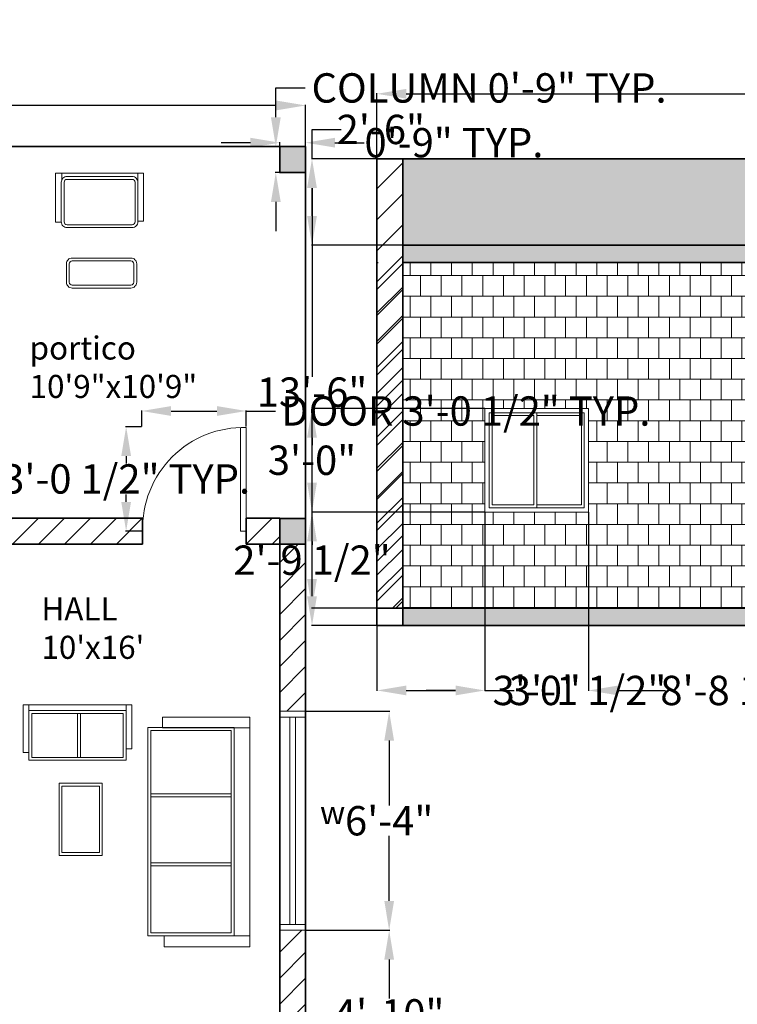
# Model space of a CAD drawing. Units: inches. Extents: x 1222 to 2611, y 176 to 793.
# Tile 3 of 5: x 1497 to 1746, y 433 to 775. Entities that reach past the tile are written whole.
import ezdxf

# ---------------------------------------------------------------- set-up
doc = ezdxf.new("R2010")
doc.units = ezdxf.units.IN
doc.header["$MEASUREMENT"] = 0
for name, color, linetype, lineweight in [('A-ANNO-DIMS', 2, 'Continuous', 18), ('A-ANNO-TEXT', 7, 'Continuous', 25), ('A-AREA-IDEN', 7, 'Continuous', 25), ('A-COLS', 7, 'Continuous', 35), ('A-COLS-PATT', 18, 'Continuous', 13), ('A-DOOR', 3, 'Continuous', 18), ('A-ELEV', 7, 'Continuous', 35), ('A-ELEV-GLAZ', 4, 'Continuous', 18), ('A-ELEV-PATT', 30, 'Continuous', 13), ('A-FURN', 8, 'Continuous', 18), ('A-GLAZ', 4, 'Continuous', 18), ('A-WALL', 7, 'Continuous', 35), ('A-WALL-PATT', 30, 'Continuous', 13)]:
    doc.layers.add(name, color=color, linetype=linetype, lineweight=lineweight)
doc.styles.get("Standard").update_dxf_attribs({"font": 'arial.ttf'})
doc.dimstyles.get("Standard").update_dxf_attribs({"dimtxt": 10.18, "dimasz": 10.18, "dimexe": 0.18, "dimexo": 0.0625, "dimgap": 0.09, "dimtad": 0, "dimtih": 1, "dimtoh": 1, "dimdec": 0, "dimzin": 0, "dimdsep": 46, "dimlunit": 3, "dimtxsty": 'Standard', "dimcen": 0.09, "dimadec": 0, "dimazin": 0, "dimtfac": 1, "dimtdec": 0, "dimtofl": 0, "dimtmove": 0, "dimatfit": 3, "dimfxl": 1, "dimtolj": 1, "dimtzin": 0, "dimarcsym": 0})

# ---------------------------------------------------------------- blocks, each defined once
blk = doc.blocks.new('*U6')
for p, q in [((1.5, 1.5), (1.5, 34.5)), ((1.5, 34.5), (18, 34.5)), ((18, 1.5), (18, 34.5)), ((18, 34.5), (34.5, 34.5)), ((34.5, 34.5), (34.5, 1.5)), ((18, 1.5), (1.5, 1.5)), ((34.5, 1.5), (18, 1.5))]:
    blk.add_line(p, q)
blk.add_lwpolyline([(0, 0), (0, 36), (36, 36), (36, 0)], close=True)
for points in [[(17, 33.5), (17, 2.5), (2.5, 2.5), (2.5, 33.5), (17, 33.5)], [(18, 33.5), (33.5, 33.5), (33.5, 2.5), (18, 2.5)]]:
    blk.add_lwpolyline(points)
blk = doc.blocks.new('*D9')
at = {"layer": 'A-ANNO-DIMS', "color": 0, "lineweight": -2, "transparency": 16777216}
for p, q in [((1328.8, 730.54), (1328.8, 744.93)), ((1338.98, 744.75), (1444.64, 744.75)), ((1585.62, 744.75), (1479.97, 744.75)), ((1595.8, 730.54), (1595.8, 744.93))]:
    blk.add_line(p, q, dxfattribs=at)
at = {"layer": 'A-ANNO-DIMS', "color": 0, "transparency": 16777216}
for points in [[(1338.98, 746.45), (1338.98, 743.05), (1328.8, 744.75)], [(1585.62, 746.45), (1585.62, 743.05), (1595.8, 744.75)]]:
    blk.add_solid(points, dxfattribs=at)
at = {"layer": 'Defpoints', "color": 0, "transparency": 16777216}
for p in [(1595.8, 744.75), (1328.8, 730.47), (1595.8, 730.47)]:
    blk.add_point(p, dxfattribs=at)
at = {"layer": 'A-ANNO-DIMS', "color": 0, "transparency": 16777216, "insert": (1462.3, 744.75), "char_height": 10.18, "attachment_point": 5}
blk.add_mtext('\\A1;22\'-3"', dxfattribs=at)
blk = doc.blocks.new('DOOR-SWING-36IN')
for p, q in [((34.01, 0), (34.01, 36)), ((36.01, 0), (36.01, 36)), ((34.01, 0), (36.01, 0))]:
    blk.add_line(p, q)
blk.add_arc((35.01, 1), 35.01, 88.3634, 181.6366)
blk = doc.blocks.new('COLUMN-9X9IN')
blk.add_lwpolyline([(0, 9), (9, 9), (9, 0), (0, 0)], close=True)
blk = doc.blocks.new('*D16')
at = {"layer": 'A-ANNO-DIMS', "color": 0, "lineweight": -2, "transparency": 16777216}
for p, q in [((1585.45, 740.65), (1585.45, 750.83)), ((1585.45, 750.83), (1595.63, 750.83)), ((1586.74, 730.47), (1585.27, 730.47)), ((1586.74, 721.47), (1585.27, 721.47)), ((1585.45, 711.29), (1585.45, 701.11))]:
    blk.add_line(p, q, dxfattribs=at)
at = {"layer": 'A-ANNO-DIMS', "color": 0, "transparency": 16777216}
for points in [[(1583.76, 740.65), (1587.15, 740.65), (1585.45, 730.47)], [(1583.76, 711.29), (1587.15, 711.29), (1585.45, 721.47)]]:
    blk.add_solid(points, dxfattribs=at)
at = {"layer": 'Defpoints', "color": 0, "transparency": 16777216}
for p in [(1585.45, 730.47), (1586.8, 730.47), (1586.8, 721.47)]:
    blk.add_point(p, dxfattribs=at)
at = {"layer": 'A-ANNO-DIMS', "color": 0, "transparency": 16777216, "insert": (1659.48, 750.83), "char_height": 10.18, "attachment_point": 5}
blk.add_mtext('\\A1;COLUMN 0\'-9" TYP.', dxfattribs=at)
blk = doc.blocks.new('*D17')
at = {"layer": 'A-ANNO-DIMS', "color": 0, "lineweight": -2, "transparency": 16777216}
for p, q in [((1576.62, 731.82), (1566.44, 731.82)), ((1586.8, 730.54), (1586.8, 732)), ((1595.8, 730.54), (1595.8, 732)), ((1605.98, 731.82), (1616.16, 731.82))]:
    blk.add_line(p, q, dxfattribs=at)
at = {"layer": 'A-ANNO-DIMS', "color": 0, "transparency": 16777216}
for points in [[(1576.62, 733.52), (1576.62, 730.13), (1586.8, 731.82)], [(1605.98, 733.52), (1605.98, 730.13), (1595.8, 731.82)]]:
    blk.add_solid(points, dxfattribs=at)
at = {"layer": 'Defpoints', "color": 0, "transparency": 16777216}
for p in [(1595.8, 731.82), (1586.8, 730.47), (1595.8, 730.47)]:
    blk.add_point(p, dxfattribs=at)
at = {"layer": 'A-ANNO-DIMS', "color": 0, "transparency": 16777216, "insert": (1647.28, 731.82), "char_height": 10.18, "attachment_point": 5}
blk.add_mtext('\\A1;0\'-9" TYP.', dxfattribs=at)
blk = doc.blocks.new('*D20')
at = {"layer": 'A-ANNO-DIMS', "color": 0, "lineweight": -2, "transparency": 16777216}
for p, q in [((1538.92, 633.31), (1538.92, 638.87)), ((1549.1, 638.69), (1565.02, 638.69)), ((1575.2, 633.31), (1575.2, 638.87)), ((1575.2, 638.69), (1585.38, 638.69))]:
    blk.add_line(p, q, dxfattribs=at)
at = {"layer": 'A-ANNO-DIMS', "color": 0, "transparency": 16777216}
for points in [[(1549.1, 640.39), (1549.1, 636.99), (1538.92, 638.69)], [(1565.02, 640.39), (1565.02, 636.99), (1575.2, 638.69)]]:
    blk.add_solid(points, dxfattribs=at)
at = {"layer": 'Defpoints', "color": 0, "transparency": 16777216}
for p in [(1575.2, 638.69), (1538.92, 633.25), (1575.2, 633.25)]:
    blk.add_point(p, dxfattribs=at)
at = {"layer": 'A-ANNO-DIMS', "color": 0, "transparency": 16777216, "insert": (1651.41, 638.69), "char_height": 10.18, "attachment_point": 5}
blk.add_mtext('\\A1;DOOR 3\'-0 1/2" TYP.', dxfattribs=at)
blk = doc.blocks.new('*D21')
at = {"layer": 'A-ANNO-DIMS', "color": 0, "lineweight": -2, "transparency": 16777216}
for p, q in [((1538.86, 633.25), (1533.3, 633.25)), ((1533.48, 623.07), (1533.48, 620.47)), ((1533.48, 607.15), (1533.48, 609.75)), ((1538.86, 596.97), (1533.3, 596.97))]:
    blk.add_line(p, q, dxfattribs=at)
at = {"layer": 'A-ANNO-DIMS', "color": 0, "transparency": 16777216}
for points in [[(1531.79, 623.07), (1535.18, 623.07), (1533.48, 633.25)], [(1531.79, 607.15), (1535.18, 607.15), (1533.48, 596.97)]]:
    blk.add_solid(points, dxfattribs=at)
at = {"layer": 'Defpoints', "color": 0, "transparency": 16777216}
for p in [(1533.48, 633.25), (1538.92, 633.25), (1538.92, 596.97)]:
    blk.add_point(p, dxfattribs=at)
at = {"layer": 'A-ANNO-DIMS', "color": 0, "transparency": 16777216, "insert": (1533.48, 615.11), "char_height": 10.18, "attachment_point": 5}
blk.add_mtext('\\A1;3\'-0 1/2" TYP.', dxfattribs=at)
blk = doc.blocks.new('*D36')
at = {"layer": 'A-ANNO-DIMS', "color": 0, "lineweight": -2, "transparency": 16777216}
for p, q in [((1595.87, 458.47), (1624.98, 458.47)), ((1624.8, 448.29), (1624.8, 434.73)), ((1624.8, 410.59), (1624.8, 424.15)), ((1595.87, 400.41), (1624.98, 400.41))]:
    blk.add_line(p, q, dxfattribs=at)
at = {"layer": 'A-ANNO-DIMS', "color": 0, "transparency": 16777216}
for points in [[(1623.11, 448.29), (1626.5, 448.29), (1624.8, 458.47)], [(1623.11, 410.59), (1626.5, 410.59), (1624.8, 400.41)]]:
    blk.add_solid(points, dxfattribs=at)
at = {"layer": 'Defpoints', "color": 0, "transparency": 16777216}
for p in [(1595.8, 458.47), (1624.8, 458.47), (1595.8, 400.41)]:
    blk.add_point(p, dxfattribs=at)
at = {"layer": 'A-ANNO-DIMS', "color": 0, "transparency": 16777216, "insert": (1624.8, 429.44), "char_height": 10.18, "attachment_point": 5}
blk.add_mtext('\\A1;4\'-10"', dxfattribs=at)
blk = doc.blocks.new('*D37')
at = {"layer": 'A-ANNO-DIMS', "color": 0, "lineweight": -2, "transparency": 16777216}
for p, q in [((1595.87, 534.47), (1624.98, 534.47)), ((1624.8, 524.29), (1624.8, 501.76)), ((1624.8, 468.65), (1624.8, 491.19)), ((1595.87, 458.47), (1624.98, 458.47))]:
    blk.add_line(p, q, dxfattribs=at)
at = {"layer": 'A-ANNO-DIMS', "color": 0, "transparency": 16777216}
for points in [[(1623.11, 524.29), (1626.5, 524.29), (1624.8, 534.47)], [(1623.11, 468.65), (1626.5, 468.65), (1624.8, 458.47)]]:
    blk.add_solid(points, dxfattribs=at)
at = {"layer": 'Defpoints', "color": 0, "transparency": 16777216}
for p in [(1595.8, 534.47), (1624.8, 534.47), (1595.8, 458.47)]:
    blk.add_point(p, dxfattribs=at)
at = {"layer": 'A-ANNO-DIMS', "color": 0, "transparency": 16777216, "insert": (1624.8, 496.47), "char_height": 10.18, "attachment_point": 5}
blk.add_mtext('\\A1;6\'-4"', dxfattribs=at)
blk = doc.blocks.new('*D42')
at = {"layer": 'A-ANNO-DIMS', "color": 0, "lineweight": -2, "transparency": 16777216}
for p, q in [((1620.56, 726.3), (1620.56, 748.97)), ((1630.74, 748.79), (1825.48, 748.79)), ((2055.37, 748.79), (1860.63, 748.79)), ((2065.55, 726.3), (2065.55, 748.97))]:
    blk.add_line(p, q, dxfattribs=at)
at = {"layer": 'A-ANNO-DIMS', "color": 0, "transparency": 16777216}
for points in [[(1630.74, 750.49), (1630.74, 747.1), (1620.56, 748.79)], [(2055.37, 750.49), (2055.37, 747.1), (2065.55, 748.79)]]:
    blk.add_solid(points, dxfattribs=at)
at = {"layer": 'Defpoints', "color": 0, "transparency": 16777216}
for p in [(2065.55, 748.79), (1620.56, 726.24), (2065.55, 726.24)]:
    blk.add_point(p, dxfattribs=at)
at = {"layer": 'A-ANNO-DIMS', "color": 0, "transparency": 16777216, "insert": (1843.06, 748.79), "char_height": 10.18, "attachment_point": 5}
blk.add_mtext('\\A1;37\'-1"', dxfattribs=at)
blk = doc.blocks.new('*D43')
at = {"layer": 'A-ANNO-DIMS', "color": 0, "lineweight": -2, "transparency": 16777216}
for p, q in [((1620.5, 726.24), (1597.83, 726.24)), ((1598.01, 716.06), (1598.01, 650.53)), ((1598.01, 574.42), (1598.01, 639.95)), ((1620.5, 564.24), (1597.83, 564.24))]:
    blk.add_line(p, q, dxfattribs=at)
at = {"layer": 'A-ANNO-DIMS', "color": 0, "transparency": 16777216}
for points in [[(1596.31, 716.06), (1599.71, 716.06), (1598.01, 726.24)], [(1596.31, 574.42), (1599.71, 574.42), (1598.01, 564.24)]]:
    blk.add_solid(points, dxfattribs=at)
at = {"layer": 'Defpoints', "color": 0, "transparency": 16777216}
for p in [(1598.01, 726.24), (1620.56, 726.24), (1620.56, 564.24)]:
    blk.add_point(p, dxfattribs=at)
at = {"layer": 'A-ANNO-DIMS', "color": 0, "transparency": 16777216, "insert": (1598.01, 645.24), "char_height": 10.18, "attachment_point": 5}
blk.add_mtext('\\A1;13\'-6"', dxfattribs=at)
blk = doc.blocks.new('*D47')
at = {"layer": 'A-ANNO-DIMS', "color": 0, "lineweight": -2, "transparency": 16777216}
for p, q in [((1598.01, 726.24), (1598.01, 736.42)), ((1598.01, 736.42), (1608.19, 736.42)), ((1620.5, 726.24), (1597.83, 726.24)), ((1598.01, 706.42), (1598.01, 716.06)), ((1629.5, 696.24), (1597.83, 696.24))]:
    blk.add_line(p, q, dxfattribs=at)
at = {"layer": 'A-ANNO-DIMS', "color": 0, "transparency": 16777216}
for points in [[(1596.31, 716.06), (1599.71, 716.06), (1598.01, 726.24)], [(1596.31, 706.42), (1599.71, 706.42), (1598.01, 696.24)]]:
    blk.add_solid(points, dxfattribs=at)
at = {"layer": 'Defpoints', "color": 0, "transparency": 16777216}
for p in [(1598.01, 726.24), (1620.56, 726.24), (1629.56, 696.24)]:
    blk.add_point(p, dxfattribs=at)
at = {"layer": 'A-ANNO-DIMS', "color": 0, "transparency": 16777216, "insert": (1621.9, 736.42), "char_height": 10.18, "attachment_point": 5}
blk.add_mtext('\\A1;2\'-6"', dxfattribs=at)
blk = doc.blocks.new('*D48')
at = {"layer": 'A-ANNO-DIMS', "color": 0, "lineweight": -2, "transparency": 16777216}
for p, q in [((1658.04, 603.54), (1658.04, 541.51)), ((1620.56, 570.18), (1620.56, 541.51)), ((1630.74, 541.69), (1647.86, 541.69)), ((1658.04, 541.69), (1668.22, 541.69))]:
    blk.add_line(p, q, dxfattribs=at)
at = {"layer": 'A-ANNO-DIMS', "color": 0, "transparency": 16777216}
for points in [[(1630.74, 543.39), (1630.74, 540), (1620.56, 541.69)], [(1647.86, 543.39), (1647.86, 540), (1658.04, 541.69)]]:
    blk.add_solid(points, dxfattribs=at)
at = {"layer": 'Defpoints', "color": 0, "transparency": 16777216}
for p in [(1658.04, 603.6), (1620.56, 570.24), (1658.04, 541.69)]:
    blk.add_point(p, dxfattribs=at)
at = {"layer": 'A-ANNO-DIMS', "color": 0, "transparency": 16777216, "insert": (1693.7, 541.69), "char_height": 10.18, "attachment_point": 5}
blk.add_mtext('\\A1;3\'-1 1/2"', dxfattribs=at)
blk = doc.blocks.new('*D49')
at = {"layer": 'A-ANNO-DIMS', "color": 0, "lineweight": -2, "transparency": 16777216}
for p, q in [((1658.04, 603.54), (1658.04, 541.51)), ((1694.04, 603.54), (1694.04, 541.51)), ((1647.86, 541.69), (1637.68, 541.69)), ((1704.22, 541.69), (1714.4, 541.69))]:
    blk.add_line(p, q, dxfattribs=at)
at = {"layer": 'A-ANNO-DIMS', "color": 0, "transparency": 16777216}
for points in [[(1647.86, 543.39), (1647.86, 540), (1658.04, 541.69)], [(1704.22, 543.39), (1704.22, 540), (1694.04, 541.69)]]:
    blk.add_solid(points, dxfattribs=at)
at = {"layer": 'Defpoints', "color": 0, "transparency": 16777216}
for p in [(1658.04, 603.6), (1694.04, 603.6), (1694.04, 541.69)]:
    blk.add_point(p, dxfattribs=at)
at = {"layer": 'A-ANNO-DIMS', "color": 0, "transparency": 16777216, "insert": (1676.04, 541.69), "char_height": 10.18, "attachment_point": 5}
blk.add_mtext('\\A1;3\'-0"', dxfattribs=at)
blk = doc.blocks.new('*D50')
at = {"layer": 'A-ANNO-DIMS', "color": 0, "lineweight": -2, "transparency": 16777216}
for p, q in [((1798.49, 606.49), (1798.49, 541.51)), ((1694.04, 603.54), (1694.04, 541.51)), ((1704.22, 541.69), (1720.78, 541.69)), ((1788.31, 541.69), (1771.76, 541.69))]:
    blk.add_line(p, q, dxfattribs=at)
at = {"layer": 'A-ANNO-DIMS', "color": 0, "transparency": 16777216}
for points in [[(1704.22, 543.39), (1704.22, 540), (1694.04, 541.69)], [(1788.31, 543.39), (1788.31, 540), (1798.49, 541.69)]]:
    blk.add_solid(points, dxfattribs=at)
at = {"layer": 'Defpoints', "color": 0, "transparency": 16777216}
for p in [(1798.49, 606.55), (1694.04, 603.6), (1798.49, 541.69)]:
    blk.add_point(p, dxfattribs=at)
at = {"layer": 'A-ANNO-DIMS', "color": 0, "transparency": 16777216, "insert": (1746.27, 541.69), "char_height": 10.18, "attachment_point": 5}
blk.add_mtext('\\A1;8\'-8 1/2"', dxfattribs=at)
blk = doc.blocks.new('*D52')
at = {"layer": 'A-ANNO-DIMS', "color": 0, "lineweight": -2, "transparency": 16777216}
for p, q in [((1657.98, 639.6), (1597.83, 639.6)), ((1598.01, 629.42), (1598.01, 626.89)), ((1598.01, 613.78), (1598.01, 616.31)), ((1657.98, 603.6), (1597.83, 603.6))]:
    blk.add_line(p, q, dxfattribs=at)
at = {"layer": 'A-ANNO-DIMS', "color": 0, "transparency": 16777216}
for points in [[(1596.31, 629.42), (1599.71, 629.42), (1598.01, 639.6)], [(1596.31, 613.78), (1599.71, 613.78), (1598.01, 603.6)]]:
    blk.add_solid(points, dxfattribs=at)
at = {"layer": 'Defpoints', "color": 0, "transparency": 16777216}
for p in [(1598.01, 639.6), (1658.04, 639.6), (1658.04, 603.6)]:
    blk.add_point(p, dxfattribs=at)
at = {"layer": 'A-ANNO-DIMS', "color": 0, "transparency": 16777216, "insert": (1598.01, 621.6), "char_height": 10.18, "attachment_point": 5}
blk.add_mtext('\\A1;3\'-0"', dxfattribs=at)
blk = doc.blocks.new('*D53')
at = {"layer": 'A-ANNO-DIMS', "color": 0, "lineweight": -2, "transparency": 16777216}
for p, q in [((1657.98, 603.6), (1597.83, 603.6)), ((1598.01, 593.42), (1598.01, 592.28)), ((1598.01, 580.42), (1598.01, 581.57)), ((1629.5, 570.24), (1597.83, 570.24))]:
    blk.add_line(p, q, dxfattribs=at)
at = {"layer": 'A-ANNO-DIMS', "color": 0, "transparency": 16777216}
for points in [[(1596.31, 593.42), (1599.71, 593.42), (1598.01, 603.6)], [(1596.31, 580.42), (1599.71, 580.42), (1598.01, 570.24)]]:
    blk.add_solid(points, dxfattribs=at)
at = {"layer": 'Defpoints', "color": 0, "transparency": 16777216}
for p in [(1598.01, 603.6), (1658.04, 603.6), (1629.56, 570.24)]:
    blk.add_point(p, dxfattribs=at)
at = {"layer": 'A-ANNO-DIMS', "color": 0, "transparency": 16777216, "insert": (1598.01, 586.92), "char_height": 10.18, "attachment_point": 5}
blk.add_mtext('\\A1;2\'-9 1/2"', dxfattribs=at)

msp = doc.modelspace()

# ---------------------------------------------------------------- hatches: boundary and pattern name
at = {"layer": 'A-COLS-PATT'}
h = msp.add_hatch(color=256, dxfattribs=at)
h.dxf.hatch_style = 1
h.paths.add_polyline_path([(1337.8, 730.47), (1328.8, 730.47), (1328.8, 721.47), (1337.8, 721.47)])
h.paths.add_polyline_path([(1466.8, 730.47), (1457.8, 730.47), (1457.8, 721.47), (1466.8, 721.47)])
h.paths.add_polyline_path([(1595.8, 730.47), (1586.8, 730.47), (1586.8, 721.47), (1595.8, 721.47)])
h.paths.add_polyline_path([(1595.8, 601.42), (1586.8, 601.42), (1586.8, 592.42), (1595.8, 592.42)])
h.paths.add_polyline_path([(1466.8, 601.47), (1457.8, 601.47), (1457.8, 592.47), (1466.8, 592.47)])
h.paths.add_polyline_path([(1337.8, 601.47), (1328.8, 601.47), (1328.8, 592.47), (1337.8, 592.47)])
h.paths.add_polyline_path([(1337.8, 400.47), (1328.8, 400.47), (1328.8, 391.47), (1337.8, 391.47)])
h.paths.add_polyline_path([(1466.8, 400.47), (1457.8, 400.47), (1457.8, 391.47), (1466.8, 391.47)])
h.paths.add_polyline_path([(1595.8, 400.41), (1586.8, 400.41), (1586.8, 391.41), (1595.8, 391.41)])
h.paths.add_polyline_path([(1466.56, 295.47), (1457.56, 295.47), (1457.56, 286.47), (1466.56, 286.47)])
h.paths.add_polyline_path([(1595.8, 295.47), (1586.8, 295.47), (1586.8, 286.47), (1595.8, 286.47)])
h.paths.add_polyline_path([(1337.8, 295.47), (1328.8, 295.47), (1328.8, 286.47), (1337.8, 286.47)])
at = {"layer": 'A-ELEV-PATT'}
h = msp.add_hatch(dxfattribs=at)
h.set_pattern_fill('ANSI31', color=256, scale=61)
h.set_pattern_definition([(45, (-599.93, -178.2906), (-5.39169, 5.39169), [])])
h.paths.add_polyline_path([(1629.56, 726.24), (1620.56, 726.24), (1620.56, 570.24), (1629.56, 570.24)])
h = msp.add_hatch(dxfattribs=at)
h.set_pattern_fill('AR-BRSTD', color=256, scale=0.9)
h.set_pattern_definition([(0, (-599.9298, -178.2906), (0, 2.4003), []), (90, (-599.9298, -178.2906), (-3.6, 2.4003), [2.4003, -2.4003])])
h.paths.add_polyline_path([(2065.55, 696.24), (2065.55, 726.24), (1629.56, 726.24), (1629.56, 696.24)])
h = msp.add_hatch(dxfattribs=at)
h.set_pattern_fill('AR-CONC', color=256, scale=0.9)
h.set_pattern_definition([(50, (-599.93, -178.2906), (6.455342, -0.564769), [0.675, -7.425]), (355, (-599.93, -178.2906), (-1.248762, 6.769729), [0.54, -5.94]), (100.45144, (-599.392, -178.3376), (5.20658, 6.20496), [0.573662, -6.310279]), (46.1842, (-599.93, -176.4906), (9.605172, -1.489674), [1.0125, -11.1375]), (96.63564, (-599.129, -176.615), (8.411958, 8.767067), [0.860493, -9.465424]), (351.18416, (-599.93, -176.491), (8.411958, 8.767067), [0.81, -8.91]), (21, (-599.03, -176.9406), (5.372163, -3.62357), [0.675, -7.425]), (326, (-599.03, -176.9406), (2.189838, 6.52635), [0.54, -5.94]), (71.45144, (-598.582, -177.2425), (7.562001, 2.90278), [0.573662, -6.310279]), (37.5, (-599.9298, -178.2906), (0.1094387, 2.9960447), [0, -5.868, 0, -6.03, 0, -5.9625]), (7.5, (-599.9298, -178.2906), (2.367626, 3.5497054), [0, -3.438, 0, -5.733, 0, -2.2725]), (327.5, (-601.9368, -178.2906), (4.804402, -0.2029938), [0, -2.25, 0, -7.02, 0, -9.315]), (317.5, (-602.837, -178.2906), (5.2486755, 0.900945), [0, -2.925, 0, -4.662, 0, -6.615])])
h.paths.add_polyline_path([(1926.91, 690.24), (2065.55, 690.24), (2065.55, 696.24), (1629.56, 696.24), (1629.56, 690.24)])
h.paths.add_polyline_path([(1629.56, 570.24), (1629.56, 564.24), (2065.55, 564.24), (2065.55, 570.24), (2007.5, 570.24), (2006.95, 569.97), (2006.81, 570.24)])
h = msp.add_hatch(dxfattribs=at)
h.set_pattern_fill('ANSI31', color=256, scale=51)
h.set_pattern_definition([(45, (-599.93, -178.2906), (-4.507806, 4.507806), [])])
h.paths.add_polyline_path([(1629.56, 690.24), (1620.56, 690.24), (1620.56, 570.24), (1629.56, 570.24)])
h.paths.add_polyline_path([(1934.74, 690.24), (1926.91, 690.24), (1926.91, 570.24), (1934.74, 570.24)])
h = msp.add_hatch(dxfattribs=at)
h.set_pattern_fill('AR-B88', color=256, scale=0.9)
h.set_pattern_definition([(0, (-599.93, -178.2906), (0, 7.2), []), (90, (-599.9298, -178.2906), (-3.6, 7.2), [7.2, -7.2])])
h.paths.add_polyline_path([(1629.56, 690.24), (1629.56, 570.24), (1926.91, 570.24), (1926.91, 690.24)])
h.paths.add_polyline_path([(1798.49, 660.55), (1858.49, 660.55), (1858.49, 606.55), (1798.49, 606.55)], flags=16)
h.paths.add_polyline_path([(1799.99, 659.05), (1828.49, 659.05), (1856.99, 659.05), (1856.99, 608.05), (1828.49, 608.05), (1799.99, 608.05)], flags=0)
h.paths.add_polyline_path([(1827.49, 609.05), (1827.49, 658.05), (1800.99, 658.05), (1800.99, 609.05)], flags=0)
h.paths.add_polyline_path([(1694.04, 639.6), (1694.04, 603.6), (1658.04, 603.6), (1658.04, 639.6)], flags=16)
h.paths.add_polyline_path([(1692.54, 638.1), (1692.54, 605.1), (1676.04, 605.1), (1659.54, 605.1), (1659.54, 638.1), (1676.04, 638.1)], flags=0)
h.paths.add_polyline_path([(1675.04, 606.1), (1675.04, 637.1), (1660.54, 637.1), (1660.54, 606.1)], flags=0)
h.paths.add_polyline_path([(1828.49, 658.05), (1855.99, 658.05), (1855.99, 609.05), (1828.49, 609.05)], flags=0)
h.paths.add_polyline_path([(1691.54, 637.1), (1691.54, 606.1), (1676.04, 606.1), (1676.04, 637.1)], flags=0)
at = {"layer": 'A-WALL-PATT'}
h = msp.add_hatch(dxfattribs=at)
h.set_pattern_fill('ANSI31', color=256, scale=51)
h.paths.add_polyline_path([(1337.8, 721.47), (1328.8, 721.47), (1328.8, 687.47), (1337.8, 687.47)])
h.paths.add_polyline_path([(1337.8, 635.47), (1328.8, 635.47), (1328.8, 601.47), (1337.8, 601.47)])
h.paths.add_polyline_path([(1371.8, 730.47), (1337.8, 730.47), (1337.8, 721.47), (1371.8, 721.47)])
h.paths.add_polyline_path([(1457.8, 730.47), (1423.8, 730.47), (1423.8, 721.47), (1457.8, 721.47)])
h.paths.add_polyline_path([(1466.8, 721.47), (1457.8, 721.47), (1457.8, 601.47), (1466.8, 601.47)])
h.paths.add_polyline_path([(1539.2, 596.97, -0.014283), (1539.2, 598.97), (1539.2, 601.47), (1466.8, 601.47), (1466.8, 592.47), (1539.2, 592.47)])
h.paths.add_polyline_path([(1595.8, 592.42), (1586.8, 592.42), (1586.8, 534.47), (1595.8, 534.47)])
h.paths.add_polyline_path([(1595.8, 458.47), (1586.8, 458.47), (1586.8, 400.41), (1595.8, 400.41)])
h.paths.add_polyline_path([(1595.8, 391.41), (1586.8, 391.41), (1586.8, 369.47), (1595.8, 369.47)])
h.paths.add_polyline_path([(1595.8, 317.47), (1586.8, 317.47), (1586.8, 295.47), (1595.8, 295.47)])
h.paths.add_polyline_path([(1586.8, 295.47), (1552.8, 295.47), (1552.8, 286.47), (1586.8, 286.47)])
h.paths.add_polyline_path([(1500.8, 295.47), (1466.8, 295.47), (1466.8, 349.72), (1462.3, 349.72, -0.014283), (1460.3, 349.72), (1457.8, 349.72), (1457.8, 295.47), (1466.56, 295.47), (1466.56, 286.47), (1500.8, 286.47)])
h.paths.add_polyline_path([(1457.56, 295.47), (1337.8, 295.47), (1337.8, 286.47), (1457.56, 286.47)])
h.paths.add_polyline_path([(1337.8, 317.47), (1328.8, 317.47), (1328.8, 295.47), (1337.8, 295.47)])
h.paths.add_polyline_path([(1337.8, 391.47), (1328.8, 391.47), (1328.8, 369.47), (1337.8, 369.47)])
h.paths.add_polyline_path([(1337.8, 434.47), (1328.8, 434.47), (1328.8, 400.47), (1337.8, 400.47)])
h.paths.add_polyline_path([(1457.8, 400.47), (1337.8, 400.47), (1337.8, 391.47), (1457.8, 391.47)])
h.paths.add_polyline_path([(1546.8, 395.97, -0.014283), (1546.8, 397.97), (1546.8, 400.47), (1466.8, 400.47), (1466.8, 391.47), (1546.8, 391.47)])
h.paths.add_polyline_path([(1466.8, 408.77), (1457.8, 408.77), (1457.8, 400.47), (1466.8, 400.47)])
h.paths.add_polyline_path([(1466.8, 391.47), (1457.8, 391.47), (1457.8, 385.72), (1466.8, 385.72)])
h.paths.add_polyline_path([(1586.8, 400.47), (1582.8, 400.47), (1582.8, 395.97), (1582.8, 391.47), (1586.8, 391.47)])
h.paths.add_polyline_path([(1466.8, 529.47), (1457.8, 529.47), (1406.8, 529.47), (1406.8, 592.47), (1414.87, 592.47), (1414.87, 596.97, -0.014283), (1414.87, 598.97), (1414.87, 601.47), (1375.45, 601.47), (1375.45, 598.97, -0.017236), (1375.45, 596.97), (1375.45, 592.47), (1397.8, 592.47), (1397.8, 529.47), (1337.8, 529.47), (1337.8, 546.97), (1328.8, 546.97), (1328.8, 486.47), (1337.8, 486.47), (1337.8, 490.02), (1337.8, 520.47), (1457.8, 520.47), (1457.8, 444.77), (1460.3, 444.77, -0.014283), (1462.3, 444.77), (1466.8, 444.77)])
h.paths.add_polyline_path([(1457.8, 601.47), (1450.87, 601.47), (1450.87, 596.97), (1450.87, 592.47), (1457.8, 592.47)], flags=0)
h.paths.add_polyline_path([(1586.8, 601.47), (1575.2, 601.47), (1575.2, 596.97), (1575.2, 592.47), (1586.8, 592.47)])

# ---------------------------------------------------------------- linework, layer by layer
at = {"layer": 'A-ELEV'}
for p, q in [((1620.56, 564.24), (1620.56, 726.24)), ((1620.56, 726.24), (2065.55, 726.24)), ((1629.56, 564.24), (1629.56, 726.24)), ((1629.56, 696.24), (2065.55, 696.24)), ((1629.56, 690.24), (1926.91, 690.24)), ((1620.56, 570.24), (1629.56, 570.24)), ((1629.56, 570.24), (2065.55, 570.24)), ((1620.56, 564.24), (2065.55, 564.24))]:
    msp.add_line(p, q, dxfattribs=at)
at = {"layer": 'A-FURN'}
for p, q in [((1516.59, 533.68), (1516.59, 518.48)), ((1517.59, 533.68), (1517.59, 518.48)), ((1542.01, 505.76), (1569.99, 505.76)), ((1542.01, 504.76), (1569.99, 504.76)), ((1542.01, 481.86), (1569.99, 481.86)), ((1542.01, 480.86), (1569.99, 480.86))]:
    msp.add_line(p, q, dxfattribs=at)
for points in [[(1511.15, 718.93), (1511.15, 721.2), (1511.15, 721.2), (1508.94, 721.2), (1508.94, 721.2), (1508.94, 704.22), (1508.94, 704.22), (1510.96, 704.22)], [(1537.37, 718.93), (1537.52, 718.93), (1537.52, 718.93), (1537.52, 721.2), (1537.52, 721.2), (1511.15, 721.2), (1511.15, 721.2), (1511.15, 718.93)]]:
    msp.add_lwpolyline(points, dxfattribs=at)
for points in [[(1537.52, 721.2), (1537.52, 721.2), (1539.56, 721.2), (1539.56, 721.2), (1539.56, 704.55), (1539.56, 704.55), (1537.52, 704.55), (1537.52, 704.55)], [(1499.7, 536.66), (1499.7, 536.66), (1497.78, 536.66), (1497.78, 536.66), (1497.78, 520.17), (1497.78, 520.17), (1499.7, 520.17), (1499.7, 520.17)], [(1499.7, 534.68), (1499.7, 534.68), (1533.5, 534.68), (1533.5, 534.68), (1533.5, 536.66), (1533.5, 536.66), (1499.7, 536.66), (1499.7, 536.66)], [(1533.5, 536.66), (1533.5, 536.66), (1535.49, 536.66), (1535.49, 536.66), (1535.49, 521.46), (1535.49, 521.46), (1533.5, 521.46), (1533.5, 521.46)], [(1499.7, 534.68), (1533.48, 534.68), (1533.48, 517.48), (1499.7, 517.48)], [(1500.7, 533.68), (1500.7, 533.68), (1532.48, 533.68), (1532.48, 533.68), (1532.48, 518.48), (1532.48, 518.48), (1500.7, 518.48), (1500.7, 518.48)], [(1576.39, 528.71), (1576.39, 528.71), (1546.12, 528.71), (1546.12, 528.71), (1546.12, 532.38), (1546.12, 532.38), (1576.39, 532.38), (1576.39, 532.38)], [(1570.99, 528.84), (1541.01, 528.84), (1541.01, 456.55), (1570.99, 456.55)], [(1569.99, 527.84), (1569.99, 527.84), (1542.01, 527.84), (1542.01, 527.84), (1542.01, 457.55), (1542.01, 457.55), (1569.99, 457.55), (1569.99, 457.55)], [(1570.99, 528.84), (1570.99, 528.84), (1570.99, 528.84), (1570.99, 528.84), (1570.99, 457.55), (1570.99, 457.55), (1570.99, 457.55), (1570.99, 457.55)], [(1570.99, 456.55), (1570.99, 456.55), (1576.39, 456.55), (1576.39, 456.55), (1576.39, 528.71), (1576.39, 528.71), (1570.99, 528.71), (1570.99, 528.71)], [(1510.17, 509.46), (1510.17, 509.46), (1525.2, 509.46), (1525.2, 509.46), (1525.2, 484.44), (1525.2, 484.44), (1510.17, 484.44), (1510.17, 484.44)], [(1511.17, 508.46), (1524.2, 508.46), (1524.2, 485.44), (1511.17, 485.44)], [(1576.39, 456.55), (1576.39, 456.55), (1546.74, 456.55), (1546.74, 456.55), (1546.74, 452.72), (1546.74, 452.72), (1576.39, 452.72), (1576.39, 452.72)]]:
    msp.add_lwpolyline(points, close=True, dxfattribs=at)
for points in [[(1510.95, 718.07, -0.414214), (1512.95, 720.07), (1535.57, 720.07, -0.414214), (1537.57, 718.07), (1537.57, 704.35, -0.414214), (1535.57, 702.35), (1512.95, 702.35, -0.414214), (1510.95, 704.35)], [(1511.95, 718.07, -0.414214), (1512.95, 719.07), (1535.57, 719.07, -0.414214), (1536.57, 718.07), (1536.57, 704.35, -0.414214), (1535.57, 703.35), (1512.95, 703.35, -0.414214), (1511.95, 704.35)], [(1512.75, 689.79, -0.414214), (1514.75, 691.79), (1535.14, 691.79, -0.414214), (1537.14, 689.79), (1537.14, 683.38, -0.414214), (1535.14, 681.38), (1514.75, 681.38, -0.414214), (1512.75, 683.38)], [(1513.75, 689.79, -0.414214), (1514.75, 690.79), (1535.14, 690.79, -0.414214), (1536.14, 689.79), (1536.14, 683.38, -0.414214), (1535.14, 682.38), (1514.75, 682.38, -0.414214), (1513.75, 683.38)]]:
    msp.add_lwpolyline(points, format="xyb", close=True, dxfattribs=at)
at = {"layer": 'A-GLAZ'}
for p, q in [((1586.8, 534.47), (1595.8, 534.47)), ((1586.8, 532.47), (1595.8, 532.47)), ((1590.3, 532.47), (1590.3, 460.47)), ((1592.3, 532.47), (1592.3, 460.47)), ((1592.3, 532.47), (1592.3, 460.47)), ((1586.8, 460.47), (1595.8, 460.47)), ((1586.8, 458.47), (1595.8, 458.47))]:
    msp.add_line(p, q, dxfattribs=at)
at = {"layer": 'A-WALL'}
for p, q in [((1328.8, 730.47), (1595.8, 730.47)), ((1595.8, 730.47), (1595.8, 286.47)), ((1466.8, 601.47), (1539.2, 601.47)), ((1539.2, 601.47), (1539.2, 592.47)), ((1575.2, 601.47), (1575.2, 592.47)), ((1575.2, 601.47), (1586.8, 601.47)), ((1466.8, 592.47), (1539.2, 592.47)), ((1575.2, 592.47), (1586.8, 592.47)), ((1586.8, 592.47), (1586.8, 400.47))]:
    msp.add_line(p, q, dxfattribs=at)

# ---------------------------------------------------------------- block references
at = {"layer": 'A-COLS'}
for p in [(1586.8, 721.47), (1586.8, 592.42)]:
    msp.add_blockref('COLUMN-9X9IN', p, dxfattribs=at)
at = {"layer": 'A-DOOR'}
msp.add_blockref('DOOR-SWING-36IN', (1539.19, 596.97), dxfattribs=at)
at = {"layer": 'A-ELEV-GLAZ'}
msp.add_blockref('*U6', (1658.04, 603.6), dxfattribs=at)

# ---------------------------------------------------------------- texts
at = {"layer": 'A-ANNO-TEXT', "insert": (1600.78, 503.29), "char_height": 8, "attachment_point": 1}
msp.add_mtext_dynamic_manual_height_columns('w', width=4.8776, gutter_width=1, heights=[0], dxfattribs=at)
at = {"layer": 'A-AREA-IDEN', "char_height": 8, "attachment_point": 1}
for s, insert in [('portico\\P10\'9"x10\'9"', (1499.96, 664.56)), ("HALL\\P10'x16'", (1504.07, 574))]:
    msp.add_mtext_dynamic_manual_height_columns(s, width=78.0148, gutter_width=1, heights=[0], dxfattribs=dict(at, insert=insert))

# ---------------------------------------------------------------- dimensions: what is measured, and where the dimension line sits
at = {"layer": 'A-ANNO-DIMS'}
for base, p1, p2, text, picture, middle in [((1585.45, 730.47), (1586.8, 721.47), (1586.8, 730.47), 'COLUMN <> TYP.', '*D16', (1659.48, 750.83)), ((1533.48, 633.25), (1538.92, 596.97), (1538.92, 633.25), '<> TYP.', '*D21', (1533.48, 615.11))]:
    dim = msp.add_linear_dim(base=base, p1=p1, p2=p2, angle=90, text=text, dimstyle='Standard', override={"dimdec": 1, "dimlfac": 1, "dimrnd": 0, "dimzin": 1, "dimdsep": 46, "dimlunit": 4, "dimfrac": 2}, dxfattribs=at)
    dim.commit()
    dim.dimension.update_dxf_attribs({"geometry": picture, "text_midpoint": middle})
for base, p1, p2, override, picture, middle in [((2065.55, 748.79), (1620.56, 726.24), (2065.55, 726.24), {"dimdec": 1, "dimlfac": 1, "dimrnd": 0, "dimzin": 1, "dimdsep": 46, "dimlunit": 4, "dimfrac": 2}, '*D42', (1843.06, 748.79)), ((1595.8, 744.75), (1328.8, 730.47), (1595.8, 730.47), {"dimclrd": 0, "dimclre": 0, "dimclrt": 0}, '*D9', (1462.3, 744.75)), ((1798.4942, 541.6919), (1694.045, 603.6028), (1798.4942, 606.5482), {"dimdec": 1, "dimlfac": 1, "dimrnd": 0, "dimzin": 1, "dimdsep": 46, "dimlunit": 4, "dimfrac": 2}, '*D50', (1746.2696, 541.6919)), ((1658.04, 541.69), (1620.56, 570.24), (1658.04, 603.6), {"dimdec": 1, "dimlfac": 1, "dimrnd": 0, "dimzin": 1, "dimdsep": 46, "dimlunit": 4, "dimfrac": 2}, '*D48', (1693.7, 541.69)), ((1694.04, 541.69), (1658.04, 603.6), (1694.04, 603.6), {"dimdec": 1, "dimlfac": 1, "dimrnd": 0, "dimzin": 1, "dimdsep": 46, "dimlunit": 4, "dimfrac": 2}, '*D49', (1676.04, 541.69))]:
    dim = msp.add_linear_dim(base=base, p1=p1, p2=p2, dimstyle='Standard', override=override, dxfattribs=at)
    dim.commit()
    dim.dimension.update_dxf_attribs({"geometry": picture, "text_midpoint": middle})
for base, p1, p2, text, picture, middle in [((1595.8, 731.82), (1586.8, 730.47), (1595.8, 730.47), '<> TYP.', '*D17', (1647.28, 731.82)), ((1575.2, 638.69), (1538.92, 633.25), (1575.2, 633.25), 'DOOR <> TYP.', '*D20', (1651.41, 638.69))]:
    dim = msp.add_linear_dim(base=base, p1=p1, p2=p2, text=text, dimstyle='Standard', override={"dimdec": 1, "dimlfac": 1, "dimrnd": 0, "dimzin": 1, "dimdsep": 46, "dimlunit": 4, "dimfrac": 2}, dxfattribs=at)
    dim.commit()
    dim.dimension.update_dxf_attribs({"geometry": picture, "text_midpoint": middle})
for base, p1, p2, picture, middle in [((1598.01, 726.24), (1629.56, 696.24), (1620.56, 726.24), '*D47', (1621.9, 736.42)), ((1598.01, 726.24), (1620.56, 564.24), (1620.56, 726.24), '*D43', (1598.01, 645.24)), ((1598.01, 639.6), (1658.04, 603.6), (1658.04, 639.6), '*D52', (1598.01, 621.6)), ((1598.01, 603.6), (1629.56, 570.24), (1658.04, 603.6), '*D53', (1598.01, 586.92)), ((1624.8, 534.47), (1595.8, 458.47), (1595.8, 534.47), '*D37', (1624.8, 496.47)), ((1624.8, 458.47), (1595.8, 400.41), (1595.8, 458.47), '*D36', (1624.8, 429.44))]:
    dim = msp.add_linear_dim(base=base, p1=p1, p2=p2, angle=90, dimstyle='Standard', override={"dimdec": 1, "dimlfac": 1, "dimrnd": 0, "dimzin": 1, "dimdsep": 46, "dimlunit": 4, "dimfrac": 2}, dxfattribs=at)
    dim.commit()
    dim.dimension.update_dxf_attribs({"geometry": picture, "text_midpoint": middle})

doc.saveas('drawing.dxf')
